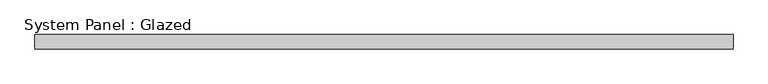
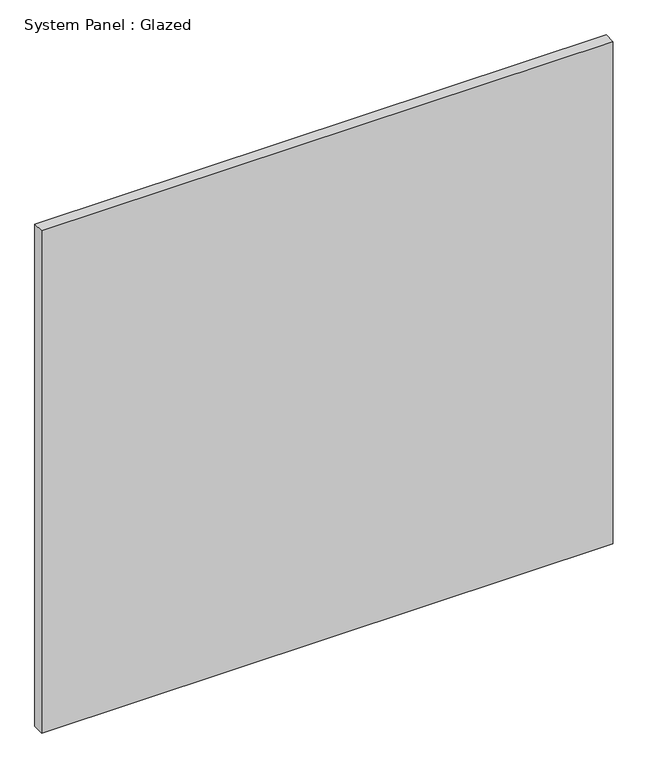
"""IFC4 building model written with IfcOpenShell, lengths in millimetres: plate geometry, System Panel : Glazed."""

from ifc_helpers import new_model, si_unit, origin, origin_with_axes, place, context, project, spatial, polyline, outline, extrude, source, transform, mapped, element, save


def system_panel_glazed_7816ce66(model_context):
    return source(origin(), model_context, "Body", "SweptSolid", [
        extrude(outline(polyline([(622.3, 19.05), (-622.3, 19.05), (-622.3, 44.45), (622.3, 44.45), (622.3, 19.05)])), origin_with_axes(), (0.0, 0.0, 1.0), 1155.7),
    ])


if __name__ == "__main__":
    model = new_model("IFC4")
    model_context = context("Model", 3, world=origin())
    ifc_project = project(units=[si_unit("LENGTHUNIT", "METRE", prefix="MILLI")], contexts=[model_context])
    site = spatial("IfcSite", under=ifc_project)
    building = spatial("IfcBuilding", under=site)
    placement = place(None, origin())
    system_panel_glazed_shape = system_panel_glazed_7816ce66(model_context)
    element("IfcPlate", 1, ObjectType="System Panel : Glazed", at=placement, inside=building, context=model_context, shape_type="MappedRepresentation", body=[
        mapped(system_panel_glazed_shape, transform((0.0, 0.0, 0.0), x_axis=(1.0, 0.0, 0.0), y_axis=(0.0, 1.0, 0.0), z_axis=(0.0, 0.0, 1.0))),
    ])
    save(model, "model.ifc")

# Revit data of these elements
# Type "System Panel : Glazed"
#   Construction Type Id = "GSP4R"
#   Analytic Construction = "1/8 in Pilkington single glazing"
#   Visual Light Transmittance = 0.9
#   Solar Heat Gain Coefficient = 0.86
#   Heat Transfer Coefficient (U) = 1.18115 BTU/(h·ft²·°F)
#   Define Thermal Properties by = 1
# Element 1 (IfcPlate, "System Panel : Glazed")
#   Materials on its faces: "Glass"
# Materials
#   "Glass": class "Glass", colour RGB 0 128 192, transparency 0.75, Description = "Soda Lime Glass", Cost = 0
